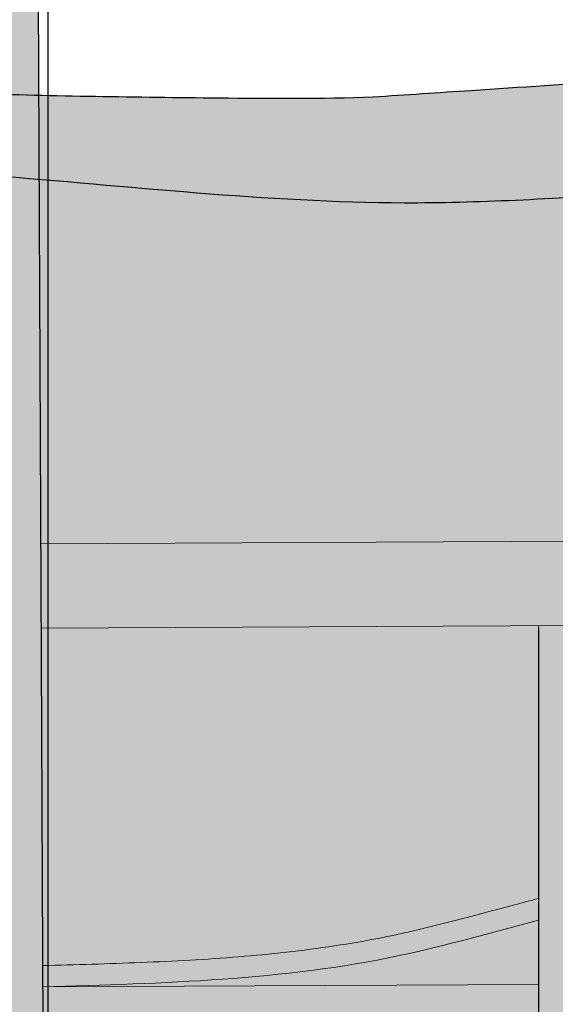
# Model space of a CAD drawing. Units: millimetres. Extents: x 11032 to 26788, y 3406 to 24505.
# Tile 65 of 78: x 18468 to 19737, y 15108 to 17443. Entities that reach past the tile are written whole.
import ezdxf

# ---------------------------------------------------------------- set-up
doc = ezdxf.new("R2010")
doc.units = ezdxf.units.MM
doc.header["$MEASUREMENT"] = 0
for name, color, linetype, lineweight in [('A-ANNO-DIMS', 2, 'Continuous', 18), ('A-ELEV-NECK', 7, 'Continuous', 25), ('A-GLAZ', 250, 'Continuous', 20), ('A-GLAZ-PATT', 9, 'Continuous', 13), ('A-ROOF', 7, 'Continuous', 30), ('E-LITE', 7, 'Continuous', 18), ('E-LITE-PATT', 7, 'Continuous', 13)]:
    doc.layers.add(name, color=color, linetype=linetype, lineweight=lineweight)
for name, color, linetype, lineweight, true_color in [('A-ELEV-NECK-PATT', 159, 'Continuous', 13, 0x22346e), ('A-GLAZ-FRAM-PATT', 250, 'Continuous', 13, 0x262627), ('A-ROOF-PATT', 9, 'Continuous', 13, 0xc7c8ca)]:
    doc.layers.add(name, color=color, linetype=linetype, lineweight=lineweight, true_color=true_color)
doc.styles.get("Standard").update_dxf_attribs({"font": 'arial.ttf'})
doc.dimstyles.get("Standard").update_dxf_attribs({"dimtxt": 150, "dimasz": 100, "dimexe": 10, "dimexo": 5, "dimgap": 5, "dimtad": 0, "dimtih": 1, "dimtoh": 1, "dimdec": 0, "dimzin": 0, "dimdsep": 46, "dimtxsty": 'Standard', "dimcen": 0.09, "dimadec": 0, "dimazin": 0, "dimtfac": 1, "dimtdec": 0, "dimtofl": 0, "dimtmove": 0, "dimatfit": 3, "dimfxl": 1, "dimtolj": 1, "dimtzin": 0, "dimarcsym": 0})

# ---------------------------------------------------------------- blocks, each defined once
blk = doc.blocks.new('*D36')
at = {"layer": 'A-ANNO-DIMS', "color": 0, "lineweight": -2, "transparency": 16777216}
for p, q in [((12301.3, 17115.9), (12301.3, 24416.9)), ((25397.4, 4466.4), (25397.4, 24416.9)), ((12401.3, 24406.9), (18569.2, 24406.9)), ((25297.4, 24406.9), (19129.5, 24406.9))]:
    blk.add_line(p, q, dxfattribs=at)
at = {"layer": 'A-ANNO-DIMS', "color": 0, "transparency": 16777216}
for points in [[(12401.3, 24423.5), (12401.3, 24390.2), (12301.3, 24406.9)], [(25297.4, 24423.5), (25297.4, 24390.2), (25397.4, 24406.9)]]:
    blk.add_solid(points, dxfattribs=at)
at = {"layer": 'Defpoints', "color": 0, "transparency": 16777216}
for p in [(25397.4, 24406.9), (12301.3, 17110.9), (25397.4, 4461.4)]:
    blk.add_point(p, dxfattribs=at)
at = {"layer": 'A-ANNO-DIMS', "color": 0, "transparency": 16777216, "insert": (18849.3, 24406.9), "char_height": 150, "attachment_point": 5}
blk.add_mtext('\\A1;13096', dxfattribs=at)
blk = doc.blocks.new('*D45')
at = {"layer": 'A-ANNO-DIMS', "color": 0, "lineweight": -2, "transparency": 16777216}
for p, q in [((13792.4, 18518.9), (26363.9, 18518.9)), ((26353.9, 18418.9), (26353.9, 17450.3)), ((26353.9, 16318.4), (26353.9, 17287)), ((22902.4, 16218.4), (26363.9, 16218.4))]:
    blk.add_line(p, q, dxfattribs=at)
at = {"layer": 'A-ANNO-DIMS', "color": 0, "transparency": 16777216}
for points in [[(26337.2, 18418.9), (26370.6, 18418.9), (26353.9, 18518.9)], [(26337.2, 16318.4), (26370.6, 16318.4), (26353.9, 16218.4)]]:
    blk.add_solid(points, dxfattribs=at)
at = {"layer": 'Defpoints', "color": 0, "transparency": 16777216}
for p in [(13787.4, 18518.9), (26353.9, 18518.9), (22897.4, 16218.4)]:
    blk.add_point(p, dxfattribs=at)
at = {"layer": 'A-ANNO-DIMS', "color": 0, "transparency": 16777216, "insert": (26353.9, 17368.7), "char_height": 150, "attachment_point": 5}
blk.add_mtext('\\A1;2300.5', dxfattribs=at)
blk = doc.blocks.new('*D50')
at = {"layer": 'A-ANNO-DIMS', "color": 0, "lineweight": -2, "transparency": 16777216}
for p, q in [((19697.4, 16000.7), (19697.4, 3494.9)), ((17953.5, 10206.4), (17953.5, 3494.9)), ((18053.5, 3504.9), (18603.8, 3504.9)), ((19597.4, 3504.9), (19047, 3504.9))]:
    blk.add_line(p, q, dxfattribs=at)
at = {"layer": 'A-ANNO-DIMS', "color": 0, "transparency": 16777216}
for points in [[(18053.5, 3521.6), (18053.5, 3488.2), (17953.5, 3504.9)], [(19597.4, 3521.6), (19597.4, 3488.2), (19697.4, 3504.9)]]:
    blk.add_solid(points, dxfattribs=at)
at = {"layer": 'Defpoints', "color": 0, "transparency": 16777216}
for p in [(19697.4, 16005.7), (17953.5, 10211.4), (19697.4, 3504.9)]:
    blk.add_point(p, dxfattribs=at)
at = {"layer": 'A-ANNO-DIMS', "color": 0, "transparency": 16777216, "insert": (18825.4, 3504.9), "char_height": 150, "attachment_point": 5}
blk.add_mtext('\\A1;1744', dxfattribs=at)
blk = doc.blocks.new('*D51')
at = {"layer": 'A-ANNO-DIMS', "color": 0, "lineweight": -2, "transparency": 16777216}
for p, q in [((19697.4, 16000.7), (19697.4, 3494.9)), ((21997.4, 16011.6), (21997.4, 3494.9)), ((19797.4, 3504.9), (20617.4, 3504.9)), ((21897.4, 3504.9), (21077.4, 3504.9))]:
    blk.add_line(p, q, dxfattribs=at)
at = {"layer": 'A-ANNO-DIMS', "color": 0, "transparency": 16777216}
for points in [[(19797.4, 3521.6), (19797.4, 3488.2), (19697.4, 3504.9)], [(21897.4, 3521.6), (21897.4, 3488.2), (21997.4, 3504.9)]]:
    blk.add_solid(points, dxfattribs=at)
at = {"layer": 'Defpoints', "color": 0, "transparency": 16777216}
for p in [(21997.4, 16016.6), (19697.4, 16005.7), (21997.4, 3504.9)]:
    blk.add_point(p, dxfattribs=at)
at = {"layer": 'A-ANNO-DIMS', "color": 0, "transparency": 16777216, "insert": (20847.4, 3504.9), "char_height": 150, "attachment_point": 5}
blk.add_mtext('\\A1;2300', dxfattribs=at)
blk = doc.blocks.new('*D57')
at = {"layer": 'A-ANNO-DIMS', "color": 0, "lineweight": -2, "transparency": 16777216}
for p, q in [((14994.7, 7266.4), (14994.7, 24416.9)), ((20894.7, 7266.4), (20894.7, 24416.9)), ((15094.7, 24406.9), (17716, 24406.9)), ((20794.7, 24406.9), (18173.4, 24406.9))]:
    blk.add_line(p, q, dxfattribs=at)
at = {"layer": 'A-ANNO-DIMS', "color": 0, "transparency": 16777216}
for points in [[(15094.7, 24423.5), (15094.7, 24390.2), (14994.7, 24406.9)], [(20794.7, 24423.5), (20794.7, 24390.2), (20894.7, 24406.9)]]:
    blk.add_solid(points, dxfattribs=at)
at = {"layer": 'Defpoints', "color": 0, "transparency": 16777216}
for p in [(20894.7, 24406.9), (14994.7, 7261.4), (20894.7, 7261.4)]:
    blk.add_point(p, dxfattribs=at)
at = {"layer": 'A-ANNO-DIMS', "color": 0, "transparency": 16777216, "insert": (17944.7, 24406.9), "char_height": 150, "attachment_point": 5}
blk.add_mtext('\\A1;5900', dxfattribs=at)
blk = doc.blocks.new('*D65')
at = {"layer": 'A-ANNO-DIMS', "color": 0, "lineweight": -2, "transparency": 16777216}
for p, q in [((17362, 12566.3), (17362, 24416.9)), ((18535.4, 12566.5), (18535.4, 24416.9)), ((17462, 24406.9), (17639.4, 24406.9)), ((18435.4, 24406.9), (18258, 24406.9))]:
    blk.add_line(p, q, dxfattribs=at)
at = {"layer": 'A-ANNO-DIMS', "color": 0, "transparency": 16777216}
for points in [[(17462, 24423.5), (17462, 24390.2), (17362, 24406.9)], [(18435.4, 24423.5), (18435.4, 24390.2), (18535.4, 24406.9)]]:
    blk.add_solid(points, dxfattribs=at)
at = {"layer": 'Defpoints', "color": 0, "transparency": 16777216}
for p in [(18535.4, 24406.9), (17362, 12561.3), (18535.4, 12561.5)]:
    blk.add_point(p, dxfattribs=at)
at = {"layer": 'A-ANNO-DIMS', "color": 0, "transparency": 16777216, "insert": (17948.7, 24406.9), "char_height": 150, "attachment_point": 5}
blk.add_mtext('\\A1;1173.3', dxfattribs=at)

msp = doc.modelspace()

# ---------------------------------------------------------------- hatches: boundary and pattern name
at = {"layer": 'A-ELEV-NECK-PATT'}
h = msp.add_hatch(color=256, dxfattribs=at)
h.set_gradient(color1=(82, 15, 16), color2=(153, 76, 0), name='INVHEMISPHERICAL')
edge = h.paths.add_edge_path()
edge.add_line((18055.913, 21712.945), (17991.118, 21712.945))
edge.add_line((17991.118, 21712.945), (17913.235, 17287.655))
edge.add_spline(control_points=[(17913.235, 17287.655), (17923.7, 17287.302), (17934.19, 17286.996), (17944.704, 17286.735)], knot_values=[8963.99017486, 8963.99017486, 8963.99017486, 8963.99017486, 8996.4318779, 8996.4318779, 8996.4318779, 8996.4318779], degree=3, periodic=0)
edge.add_spline(control_points=[(17944.704, 17286.735), (17964.82, 17285.722), (17984.935, 17284.709), (18005.051, 17283.703)], knot_values=[0, 0, 0, 0, 60.41749209, 60.41749209, 60.41749209, 60.41749209], degree=3, periodic=0)
edge.add_line((18005.051, 17283.703), (18055.913, 21712.945))
edge = h.paths.add_edge_path()
edge.add_line((18492.19, 21712.945), (18416.998, 21712.945))
edge.add_line((18416.998, 21712.945), (18420.504, 17266.134))
edge.add_spline(control_points=[(18420.504, 17266.134), (18451.394, 17265.216), (18482.287, 17264.397), (18513.182, 17263.662)], knot_values=[476.26006783, 476.26006783, 476.26006783, 476.26006783, 568.98430855, 568.98430855, 568.98430855, 568.98430855], degree=3, periodic=0)
edge.add_line((18513.182, 17263.662), (18492.19, 21712.945))
edge = h.paths.add_edge_path()
edge.add_spline(control_points=[(18296.914, 17270.367), (18316.656, 17269.603), (18349.518, 17268.396), (18382.383, 17267.313), (18395.503, 17266.9)], knot_values=[352.58081587, 352.58081587, 352.58081587, 352.58081587, 411.85892504, 451.24395945, 451.24395945, 451.24395945, 451.24395945], degree=3, periodic=0)
edge.add_line((18395.503, 17266.9), (18391.999, 21712.945))
edge.add_line((18391.999, 21712.945), (18316.752, 21712.945))
edge.add_line((18316.752, 21712.945), (18296.914, 17270.367))
edge = h.paths.add_edge_path()
edge.add_line((18291.755, 21712.945), (18216.518, 21712.945))
edge.add_line((18216.518, 21712.945), (18173.381, 17275.594))
edge.add_spline(control_points=[(18173.381, 17275.594), (18206.225, 17274.101), (18239.071, 17272.678), (18271.92, 17271.355)], knot_values=[228.93242669, 228.93242669, 228.93242669, 228.93242669, 327.56540209, 327.56540209, 327.56540209, 327.56540209], degree=3, periodic=0)
edge.add_line((18271.92, 17271.355), (18291.755, 21712.945))
h = msp.add_hatch(color=256, dxfattribs=at)
h.set_gradient(color1=(153, 76, 0), color2=(153, 38, 0), name='INVSPHERICAL')
edge = h.paths.add_edge_path()
edge.add_spline(control_points=[(17641.798, 17308.706), (17605.243, 17313.31), (17568.929, 17318.668), (17532.827, 17324.837)], knot_values=[8560.66857913, 8560.66857913, 8560.66857913, 8560.66857913, 8678.18536837, 8678.18536837, 8678.18536837, 8678.18536837], degree=3, periodic=0)
edge.add_line((17532.827, 17324.837), (17525.58, 17122.709))
edge.add_spline(control_points=[(17525.58, 17122.709), (17542.498, 17119.989), (17559.438, 17117.434), (17596.281, 17112.234), (17616.191, 17109.648), (17636.137, 17107.272)], knot_values=[8357.5016646, 8357.5016646, 8357.5016646, 8357.5016646, 8408.27359921, 8408.27359921, 8467.76262378, 8467.76262378, 8467.76262378, 8467.76262378], degree=3, periodic=0)
edge.add_line((17636.137, 17107.272), (17641.798, 17308.706))
edge = h.paths.add_edge_path()
edge.add_spline(control_points=[(17764.917, 17296.043), (17731.975, 17298.702), (17699.249, 17301.903), (17666.718, 17305.687)], knot_values=[8704.84912349, 8704.84912349, 8704.84912349, 8704.84912349, 8809.1081873, 8809.1081873, 8809.1081873, 8809.1081873], degree=3, periodic=0)
edge.add_line((17666.718, 17305.687), (17661.061, 17104.414))
edge.add_spline(control_points=[(17661.061, 17104.414), (17679.29, 17102.404), (17697.549, 17100.566), (17730.647, 17097.538), (17745.476, 17096.292), (17760.326, 17095.15)], knot_values=[8492.52413318, 8492.52413318, 8492.52413318, 8492.52413318, 8546.81227116, 8546.81227116, 8590.76516304, 8590.76516304, 8590.76516304, 8590.76516304], degree=3, periodic=0)
edge.add_line((17760.326, 17095.15), (17764.917, 17296.043))
edge = h.paths.add_edge_path()
edge.add_spline(control_points=[(17785.288, 17093.328), (17818.317, 17091.049), (17851.456, 17089.272), (17884.718, 17087.959)], knot_values=[8615.37173025, 8615.37173025, 8615.37173025, 8615.37173025, 8712.96274361, 8712.96274361, 8712.96274361, 8712.96274361], degree=3, periodic=0)
edge.add_line((17884.718, 17087.959), (17888.249, 17288.59))
edge.add_spline(control_points=[(17888.249, 17288.59), (17855.23, 17289.947), (17822.446, 17291.782), (17789.878, 17294.135)], knot_values=[8835.39626479, 8835.39626479, 8835.39626479, 8835.39626479, 8938.12522047, 8938.12522047, 8938.12522047, 8938.12522047], degree=3, periodic=0)
edge.add_line((17789.878, 17294.135), (17785.288, 17093.328))
edge = h.paths.add_edge_path()
edge.add_spline(control_points=[(17909.705, 17087.059), (17910.273, 17087.04), (17910.841, 17087.022), (17922.493, 17086.648), (17933.591, 17086.342), (17944.704, 17086.084)], knot_values=[8737.37614655, 8737.37614655, 8737.37614655, 8737.37614655, 8739.04043473, 8739.04043473, 8771.49406906, 8771.49406906, 8771.49406906, 8771.49406906], degree=3, periodic=0)
edge.add_spline(control_points=[(17944.704, 17086.084), (17964.06, 17086.958), (17983.426, 17087.583), (18002.804, 17087.985)], knot_values=[1891.03799383, 1891.03799383, 1891.03799383, 1891.03799383, 1949.25960113, 1949.25960113, 1949.25960113, 1949.25960113], degree=3, periodic=0)
edge.add_line((18002.804, 17087.985), (18005.051, 17283.703))
edge.add_spline(control_points=[(18005.051, 17283.703), (17984.935, 17284.709), (17964.82, 17285.722), (17944.704, 17286.735)], knot_values=[0, 0, 0, 0, 60.41749209, 60.41749209, 60.41749209, 60.41749209], degree=3, periodic=0)
edge.add_spline(control_points=[(17944.704, 17286.735), (17934.19, 17286.996), (17923.7, 17287.302), (17913.235, 17287.655)], knot_values=[8963.99017486, 8963.99017486, 8963.99017486, 8963.99017486, 8996.4318779, 8996.4318779, 8996.4318779, 8996.4318779], degree=3, periodic=0)
edge.add_line((17913.235, 17287.655), (17909.705, 17087.059))
edge = h.paths.add_edge_path()
edge.add_spline(control_points=[(18148.395, 17276.742), (18108.941, 17278.575), (18069.489, 17280.497), (18030.038, 17282.457)], knot_values=[85.43243603, 85.43243603, 85.43243603, 85.43243603, 203.92020001, 203.92020001, 203.92020001, 203.92020001], degree=3, periodic=0)
edge.add_line((18030.038, 17282.457), (18027.809, 17088.381))
edge.add_spline(control_points=[(18027.809, 17088.381), (18067.33, 17088.817), (18106.905, 17088.367), (18146.553, 17087.237)], knot_values=[1747.32517671, 1747.32517671, 1747.32517671, 1747.32517671, 1866.00187039, 1866.00187039, 1866.00187039, 1866.00187039], degree=3, periodic=0)
edge.add_line((18146.553, 17087.237), (18148.395, 17276.742))
edge = h.paths.add_edge_path()
edge.add_spline(control_points=[(18271.92, 17271.355), (18239.071, 17272.678), (18206.225, 17274.101), (18173.381, 17275.594)], knot_values=[228.93242669, 228.93242669, 228.93242669, 228.93242669, 327.56540209, 327.56540209, 327.56540209, 327.56540209], degree=3, periodic=0)
edge.add_line((18173.381, 17275.594), (18171.542, 17086.437))
edge.add_spline(control_points=[(18171.542, 17086.437), (18204.662, 17085.263), (18237.835, 17083.647), (18271.073, 17081.706)], knot_values=[1623.3453903, 1623.3453903, 1623.3453903, 1623.3453903, 1722.40133721, 1722.40133721, 1722.40133721, 1722.40133721], degree=3, periodic=0)
edge.add_line((18271.073, 17081.706), (18271.92, 17271.355))
edge = h.paths.add_edge_path()
edge.add_spline(control_points=[(18296.064, 17080.189), (18329.191, 17078.104), (18362.384, 17075.728), (18395.656, 17073.18)], knot_values=[1499.9078295, 1499.9078295, 1499.9078295, 1499.9078295, 1598.53123513, 1598.53123513, 1598.53123513, 1598.53123513], degree=3, periodic=0)
edge.add_line((18395.656, 17073.18), (18395.503, 17266.9))
edge.add_spline(control_points=[(18395.503, 17266.9), (18382.383, 17267.313), (18349.518, 17268.396), (18316.656, 17269.603), (18296.914, 17270.367)], knot_values=[352.58081587, 352.58081587, 352.58081587, 352.58081587, 391.96585028, 451.24395945, 451.24395945, 451.24395945, 451.24395945], degree=3, periodic=0)
edge.add_line((18296.914, 17270.367), (18296.064, 17080.189))
edge = h.paths.add_edge_path()
edge.add_spline(control_points=[(18420.658, 17071.235), (18423.571, 17071.005), (18454.665, 17068.542), (18485.83, 17065.963), (18514.126, 17063.566)], knot_values=[1383.18424693, 1383.18424693, 1383.18424693, 1383.18424693, 1391.81011968, 1475.21962479, 1475.21962479, 1475.21962479, 1475.21962479], degree=3, periodic=0)
edge.add_line((18514.126, 17063.566), (18513.182, 17263.662))
edge.add_spline(control_points=[(18513.182, 17263.662), (18482.287, 17264.397), (18451.394, 17265.216), (18420.504, 17266.134)], knot_values=[476.26006783, 476.26006783, 476.26006783, 476.26006783, 568.98430855, 568.98430855, 568.98430855, 568.98430855], degree=3, periodic=0)
edge.add_line((18420.504, 17266.134), (18420.658, 17071.235))
h = msp.add_hatch(color=256, dxfattribs=at)
h.set_gradient(color1=(82, 15, 16), color2=(153, 76, 0), name='INVHEMISPHERICAL')
edge = h.paths.add_edge_path()
edge.add_line((17829.868, 12550.781), (17950.703, 12550.781))
edge.add_line((17950.703, 12550.781), (18002.804, 17087.985))
edge.add_spline(control_points=[(18002.804, 17087.985), (17983.426, 17087.583), (17964.06, 17086.958), (17944.704, 17086.084)], knot_values=[1891.03799383, 1891.03799383, 1891.03799383, 1891.03799383, 1949.25960113, 1949.25960113, 1949.25960113, 1949.25960113], degree=3, periodic=0)
edge.add_spline(control_points=[(17944.704, 17086.084), (17933.591, 17086.342), (17922.493, 17086.648), (17910.841, 17087.022), (17910.273, 17087.04), (17909.705, 17087.059)], knot_values=[8737.37614655, 8737.37614655, 8737.37614655, 8737.37614655, 8769.82978089, 8769.82978089, 8771.49406906, 8771.49406906, 8771.49406906, 8771.49406906], degree=3, periodic=0)
edge.add_line((17909.705, 17087.059), (17829.868, 12550.781))
edge = h.paths.add_edge_path()
edge.add_spline(control_points=[(18146.553, 17087.237), (18106.905, 17088.367), (18067.33, 17088.817), (18027.809, 17088.381)], knot_values=[1747.32517671, 1747.32517671, 1747.32517671, 1747.32517671, 1866.00187039, 1866.00187039, 1866.00187039, 1866.00187039], degree=3, periodic=0)
edge.add_line((18027.809, 17088.381), (17975.703, 12550.781))
edge.add_line((17975.703, 12550.781), (18102.451, 12550.781))
edge.add_line((18102.451, 12550.781), (18146.553, 17087.237))
edge = h.paths.add_edge_path()
edge.add_line((18127.45, 12550.781), (18250.839, 12550.781))
edge.add_line((18250.839, 12550.781), (18271.073, 17081.706))
edge.add_spline(control_points=[(18271.073, 17081.706), (18237.835, 17083.647), (18204.662, 17085.263), (18171.542, 17086.437)], knot_values=[1623.3453903, 1623.3453903, 1623.3453903, 1623.3453903, 1722.40133721, 1722.40133721, 1722.40133721, 1722.40133721], degree=3, periodic=0)
edge.add_line((18171.542, 17086.437), (18127.45, 12550.781))
edge = h.paths.add_edge_path()
edge.add_spline(control_points=[(18395.656, 17073.18), (18362.384, 17075.728), (18329.191, 17078.104), (18296.064, 17080.189)], knot_values=[1499.9078295, 1499.9078295, 1499.9078295, 1499.9078295, 1598.53123513, 1598.53123513, 1598.53123513, 1598.53123513], degree=3, periodic=0)
edge.add_line((18296.064, 17080.189), (18275.839, 12550.781))
edge.add_line((18275.839, 12550.781), (18399.221, 12550.781))
edge.add_line((18399.221, 12550.781), (18395.656, 17073.18))
edge = h.paths.add_edge_path()
edge.add_spline(control_points=[(18514.126, 17063.566), (18485.83, 17065.963), (18454.665, 17068.542), (18423.571, 17071.005), (18420.658, 17071.235)], knot_values=[1383.18424693, 1383.18424693, 1383.18424693, 1383.18424693, 1466.59375204, 1475.21962479, 1475.21962479, 1475.21962479, 1475.21962479], degree=3, periodic=0)
edge.add_line((18420.658, 17071.235), (18424.221, 12551.892))
edge.add_line((18424.221, 12551.892), (18535.368, 12561.343))
edge.add_line((18535.368, 12561.343), (18514.126, 17063.566))
edge = h.paths.add_edge_path()
edge.add_spline(control_points=[(17636.137, 17107.272), (17616.191, 17109.648), (17596.281, 17112.234), (17559.438, 17117.434), (17542.498, 17119.989), (17525.58, 17122.709)], knot_values=[8357.5016646, 8357.5016646, 8357.5016646, 8357.5016646, 8416.99068917, 8416.99068917, 8467.76262378, 8467.76262378, 8467.76262378, 8467.76262378], degree=3, periodic=0)
edge.add_line((17525.58, 17122.709), (17362.033, 12561.3))
edge.add_line((17362.033, 12561.3), (17485.63, 12550.781))
edge.add_line((17485.63, 12550.781), (17508.079, 12550.781))
edge.add_line((17508.079, 12550.781), (17636.137, 17107.272))
edge = h.paths.add_edge_path()
edge.add_spline(control_points=[(17760.326, 17095.15), (17745.476, 17096.292), (17730.647, 17097.538), (17697.549, 17100.566), (17679.29, 17102.404), (17661.061, 17104.414)], knot_values=[8492.52413318, 8492.52413318, 8492.52413318, 8492.52413318, 8536.47702506, 8536.47702506, 8590.76516304, 8590.76516304, 8590.76516304, 8590.76516304], degree=3, periodic=0)
edge.add_line((17661.061, 17104.414), (17533.08, 12550.781))
edge.add_line((17533.08, 12550.781), (17656.474, 12550.781))
edge.add_line((17656.474, 12550.781), (17760.326, 17095.15))
edge = h.paths.add_edge_path()
edge.add_spline(control_points=[(17884.718, 17087.959), (17851.456, 17089.272), (17818.317, 17091.049), (17785.288, 17093.328)], knot_values=[8615.37173025, 8615.37173025, 8615.37173025, 8615.37173025, 8712.96274361, 8712.96274361, 8712.96274361, 8712.96274361], degree=3, periodic=0)
edge.add_line((17785.288, 17093.328), (17681.475, 12550.781))
edge.add_line((17681.475, 12550.781), (17804.868, 12550.781))
edge.add_line((17804.868, 12550.781), (17884.718, 17087.959))
at = {"layer": 'A-GLAZ-FRAM-PATT'}
h = msp.add_hatch(color=256, dxfattribs=at)
h.paths.add_polyline_path([(22747.404, 16218.44), (22395.025, 16218.44), (18518.2, 16200.148), (18519.143, 16000.151), (22747.404, 16020.1)])
edge = h.paths.add_edge_path()
edge.add_line((22897.404, 16218.44), (22747.404, 16218.44))
edge.add_line((22747.404, 16218.44), (22747.404, 16020.1))
edge.add_line((22747.404, 16020.1), (22747.404, 9631.346))
edge.add_spline(control_points=[(22747.404, 9631.346), (22803.273, 9520.228), (22853.467, 9405.87), (22897.404, 9289.211)], knot_values=[2645.78092422, 2645.78092422, 2645.78092422, 2645.78092422, 3013.05623672, 3013.05623672, 3013.05623672, 3013.05623672], degree=3, periodic=0)
edge.add_line((22897.404, 9289.211), (22897.404, 16218.44))
h.paths.add_polyline_path([(22097.404, 16017.033), (21997.404, 16016.562), (21997.404, 13316.532), (22097.404, 13317.003)])
edge = h.paths.add_edge_path()
edge.add_line((19797.404, 16006.182), (19697.404, 16005.71))
edge.add_line((19697.404, 16005.71), (19697.404, 15155.703))
edge.add_line((19697.404, 15155.703), (19697.404, 12747.012))
edge.add_spline(control_points=[(19697.404, 12747.012), (19708.389, 12750.081), (19719.253, 12753.406), (19732.457, 12757.789), (19734.918, 12758.62), (19737.372, 12759.464)], knot_values=[1372.60477099, 1372.60477099, 1372.60477099, 1372.60477099, 1399.44343377, 1399.44343377, 1405.61279972, 1405.61279972, 1405.61279972, 1405.61279972], degree=3, periodic=0)
edge.add_spline(control_points=[(19737.372, 12759.464), (19750.245, 12763.891), (19762.932, 12768.657), (19778.9, 12775.14), (19782.354, 12776.572), (19785.794, 12778.028)], knot_values=[1405.61279972, 1405.61279972, 1405.61279972, 1405.61279972, 1437.96891336, 1437.96891336, 1446.94640473, 1446.94640473, 1446.94640473, 1446.94640473], degree=3, periodic=0)
edge.add_spline(control_points=[(19785.794, 12778.028), (19789.682, 12779.673), (19793.552, 12781.348), (19797.404, 12783.051)], knot_values=[1446.94640473, 1446.94640473, 1446.94640473, 1446.94640473, 1457.09545574, 1457.09545574, 1457.09545574, 1457.09545574], degree=3, periodic=0)
edge.add_line((19797.404, 12783.051), (19797.404, 15306.174))
edge.add_line((19797.404, 15306.174), (19797.404, 16006.182))
h = msp.add_hatch(color=256, dxfattribs=at)
h.paths.add_polyline_path([(19697.404, 15155.703), (18523.154, 15150.163), (18523.626, 15050.164), (19697.404, 15055.702)])
h.paths.add_polyline_path([(21997.404, 15166.555), (19797.404, 15156.175), (19797.404, 15056.174), (20912.335, 15061.434, -0.11801722), (20947.253, 15061.599), (21997.404, 15066.554)])
h.paths.add_polyline_path([(22747.404, 15170.094), (22097.404, 15167.027), (22097.404, 15067.026), (22747.404, 15070.092)])
edge = h.paths.add_edge_path()
edge.add_line((21997.404, 13241.531), (21332.397, 13238.393))
edge.add_spline(control_points=[(21332.397, 13238.393), (21338.038, 13214.902), (21343.139, 13191.382), (21354.5, 13132.481), (21360.029, 13097.149), (21368.306, 13027.119), (21371.052, 12992.421), (21373.63, 12924.101), (21373.462, 12890.481), (21370.61, 12834.187), (21368.665, 12811.15), (21365.955, 12788.546)], knot_values=[4470.65028407, 4470.65028407, 4470.65028407, 4470.65028407, 4531.4505555, 4531.4505555, 4623.16319106, 4623.16319106, 4714.87582662, 4714.87582662, 4806.58846218, 4806.58846218, 4871.89074498, 4871.89074498, 4871.89074498, 4871.89074498], degree=3, periodic=0)
edge.add_line((21365.955, 12788.546), (21997.404, 12791.526))
edge.add_line((21997.404, 12791.526), (21997.404, 13241.531))
h.paths.add_polyline_path([(22097.404, 13242.003), (21997.404, 13241.531), (21997.404, 12791.526), (22097.404, 12791.998)])
h.paths.add_polyline_path([(22697.404, 13244.833), (22097.404, 13242.003), (22097.404, 12791.998), (22697.404, 12794.828)])
at = {"layer": 'A-GLAZ-PATT'}
h = msp.add_hatch(color=256, dxfattribs=at)
h.set_gradient(color1=(254, 221, 154), color2=(248, 246, 176), name='CURVED')
edge = h.paths.add_edge_path()
edge.add_spline(control_points=[(18522.918, 15200.175), (18561.599, 15201.209), (18600.224, 15202.243), (18716.594, 15205.749), (18794.099, 15208.613), (18948.086, 15217.451), (19024.568, 15223.425), (19176.135, 15240.511), (19251.219, 15251.623), (19333.848, 15267.966), (19342.25, 15269.676), (19356.967, 15272.758), (19363.289, 15274.111), (19375.94, 15276.871), (19382.267, 15278.279), (19401.252, 15282.576), (19413.915, 15285.541), (19451.935, 15294.685), (19477.322, 15301.111), (19548.254, 15319.552), (19593.948, 15331.984), (19659.079, 15349.253), (19678.203, 15354.269), (19697.404, 15359.188)], knot_values=[1.09285599, 1.09285599, 1.09285599, 1.09285599, 116.34451384, 116.34451384, 349.03354152, 349.03354152, 581.72256921, 581.72256921, 814.41159689, 814.41159689, 840.78637359, 840.78637359, 860.67891922, 860.67891922, 880.57146485, 880.57146485, 920.35655611, 920.35655611, 999.92673863, 999.92673863, 1142.09604805, 1142.09604805, 1200.90860694, 1200.90860694, 1200.90860694, 1200.90860694], degree=3, periodic=0)
edge.add_line((19697.404, 15359.188), (19697.404, 16005.71))
edge.add_line((19697.404, 16005.71), (18519.143, 16000.151))
edge.add_line((18519.143, 16000.151), (18522.918, 15200.175))
edge = h.paths.add_edge_path()
edge.add_line((19697.404, 15055.702), (18523.626, 15050.164))
edge.add_line((18523.626, 15050.164), (18531.851, 13306.733))
edge.add_spline(control_points=[(18531.851, 13306.733), (18553.325, 13284.933), (18574.901, 13263.301), (18632.771, 13206.214), (18669.261, 13171.188), (18735.852, 13109.762), (18765.813, 13083.011), (18826.398, 13031.156), (18857.021, 13006.052), (18919.15, 12957.862), (18950.655, 12934.774), (19007.615, 12895.967), (19032.834, 12879.759), (19084.165, 12849.05), (19110.278, 12834.547), (19163.6, 12807.555), (19190.811, 12795.065), (19240.068, 12775.123), (19261.85, 12767.175), (19306.233, 12752.949), (19328.834, 12746.672), (19374.859, 12736.071), (19398.283, 12731.748), (19445.866, 12725.365), (19470.026, 12723.306), (19514.597, 12721.889), (19534.921, 12722.121), (19575.756, 12724.466), (19596.267, 12726.579), (19622.683, 12730.57), (19628.6, 12731.546), (19638.601, 12733.337), (19642.688, 12734.108), (19650.826, 12735.723), (19654.881, 12736.567), (19667.001, 12739.207), (19675.023, 12741.111), (19687.813, 12744.388), (19692.62, 12745.676), (19697.404, 12747.012)], knot_values=[259.28299856, 259.28299856, 259.28299856, 259.28299856, 332.45020059, 332.45020059, 454.53383699, 454.53383699, 552.84889009, 552.84889009, 651.16394319, 651.16394319, 749.47899629, 749.47899629, 825.6298474, 825.6298474, 901.7806985, 901.7806985, 977.9315496, 977.9315496, 1036.43952646, 1036.43952646, 1094.94750331, 1094.94750331, 1153.45548017, 1153.45548017, 1211.96345702, 1211.96345702, 1260.21270617, 1260.21270617, 1308.46195531, 1308.46195531, 1322.39247458, 1322.39247458, 1332.02384448, 1332.02384448, 1341.65521438, 1341.65521438, 1360.91795418, 1360.91795418, 1372.60477099, 1372.60477099, 1372.60477099, 1372.60477099], degree=3, periodic=0)
edge.add_line((19697.404, 12747.012), (19697.404, 15055.702))
h.paths.add_polyline_path([(18790.086, 14298.34, -1), (18890.086, 14298.34, -1)], flags=16)
h.paths.add_polyline_path([(19437.524, 14550.125, -1), (19537.524, 14550.125, -1)], flags=16)
h.paths.add_polyline_path([(22697.404, 16019.864), (22097.404, 16017.033), (22097.404, 15167.027), (22697.404, 15169.858)])
h.paths.add_polyline_path([(22697.404, 15069.857), (22097.404, 15067.026), (22097.404, 13317.003), (22697.404, 13319.834)])
h.paths.add_polyline_path([(20866.429, 15795.606, -1), (21016.429, 15795.606, -1)], flags=16)
h.paths.add_polyline_path([(19822.441, 15337.78), (19797.404, 15332.147), (19797.404, 15156.175), (20721.869, 15160.537), (20700.803, 15175.665), (20679.512, 15190.548), (20657.993, 15205.143), (20636.247, 15219.41), (20614.273, 15233.307), (20592.07, 15246.794), (20569.639, 15259.829), (20546.978, 15272.372), (20524.088, 15284.38), (20500.968, 15295.814), (20477.616, 15306.631), (20454.034, 15316.792), (20430.219, 15326.254), (20406.173, 15334.976), (20381.894, 15342.919), (20357.382, 15350.039), (20332.636, 15356.297), (20307.662, 15361.667), (20282.483, 15366.173), (20257.125, 15369.849), (20231.617, 15372.729), (20205.984, 15374.847), (20180.253, 15376.236), (20154.451, 15376.931), (20128.605, 15376.964), (20102.742, 15376.37), (20076.889, 15375.183), (20051.072, 15373.436), (20025.318, 15371.163), (19999.653, 15368.398), (19974.087, 15365.173), (19948.614, 15361.516), (19923.228, 15357.456), (19897.924, 15353.024), (19872.695, 15348.248), (19847.536, 15343.157)])
h.paths.add_polyline_path([(19797.404, 15383.428), (19822.666, 15388.998), (19848.044, 15394.311), (19873.542, 15399.338), (19899.168, 15404.048), (19924.927, 15408.41), (19950.824, 15412.396), (19976.865, 15415.972), (20003.054, 15419.109), (20029.394, 15421.774), (20055.871, 15423.934), (20082.461, 15425.553), (20109.142, 15426.594), (20135.888, 15427.02), (20162.676, 15426.794), (20189.481, 15425.88), (20216.28, 15424.237), (20243.046, 15421.828), (20269.754, 15418.614), (20296.377, 15414.554), (20322.887, 15409.61), (20349.254, 15403.74), (20375.368, 15396.947), (20401.163, 15389.283), (20426.64, 15380.795), (20451.799, 15371.531), (20476.643, 15361.538), (20501.172, 15350.863), (20525.391, 15339.55), (20549.302, 15327.645), (20572.91, 15315.192), (20596.218, 15302.234), (20619.229, 15288.816), (20641.948, 15274.978), (20664.378, 15260.764), (20686.523, 15246.215), (20708.386, 15231.373), (20729.97, 15216.279), (20751.277, 15200.974), (20806.33, 15160.935), (21997.404, 15166.555), (21997.404, 16016.562), (19797.404, 16006.182)])
at = {"layer": 'A-ROOF-PATT'}
h = msp.add_hatch(color=256, dxfattribs=at)
edge = h.paths.add_edge_path()
edge.add_spline(control_points=[(18514.126, 17063.566), (18809.773, 17038.521), (19288.07, 16988.339), (19761.843, 17020.464), (19965.955, 17031.58)], knot_values=[0, 0, 0, 0, 871.48115533, 1383.18424693, 1383.18424693, 1383.18424693, 1383.18424693], degree=3, periodic=0)
edge.add_spline(control_points=[(19965.955, 17031.58), (20122.484, 17046.068), (20408.011, 17091.181), (20910.567, 17150.246), (21440.234, 17310.172), (21915.866, 17351.508), (22364.272, 17406.622), (22705.353, 17409.356), (22912.577, 17410.967), (22981.194, 17409.426)], knot_values=[0, 0, 0, 0, 414.81784697, 1085.22788952, 1556.54039253, 2003.31216232, 2520.51919616, 2899.47011217, 3092.27759325, 3092.27759325, 3092.27759325, 3092.27759325], degree=3, periodic=0)
edge.add_spline(control_points=[(22981.194, 17409.426), (23026.355, 17412.719), (23070.675, 17406.134), (23179.968, 17412.17), (23244.326, 17403.734), (23304.873, 17403.391)], knot_values=[11756.28081343, 11756.28081343, 11756.28081343, 11756.28081343, 11879.15309498, 11879.15309498, 12065.87545546, 12065.87545546, 12065.87545546, 12065.87545546], degree=3, periodic=0)
edge.add_spline(control_points=[(23304.873, 17403.391), (23443.416, 17391.278), (23687.5, 17400.339), (23988.629, 17323.661), (24193.084, 17226.949), (24257.37, 17136.735), (24279.347, 17098.191)], knot_values=[0, 0, 0, 0, 412.75172359, 727.19040018, 931.86025321, 1064.01641738, 1064.01641738, 1064.01641738, 1064.01641738], degree=3, periodic=0)
edge.add_spline(control_points=[(24279.347, 17098.191), (24276.632, 17112.026), (24103.56, 17784.539), (21679.83, 17482.933), (20092.886, 17311.864), (19886.51, 17298.161)], knot_values=[9435.32329041, 9435.32329041, 9435.32329041, 9435.32329041, 9511.54858978, 13244.41643911, 13837.11981978, 13837.11981978, 13837.11981978, 13837.11981978], degree=3, periodic=0)
edge.add_spline(control_points=[(19886.51, 17298.161), (19770.33, 17290.447), (19654.15, 17282.732), (19537.97, 17275.018), (19460.41, 17269.868), (19382.851, 17264.718), (19305.291, 17259.568)], knot_values=[8878.9087223, 8878.9087223, 8878.9087223, 8878.9087223, 9212.57342317, 9212.57342317, 9212.57342317, 9435.32303857, 9435.32303857, 9435.32303857, 9435.32303857], degree=3, periodic=0)
edge.add_spline(control_points=[(19305.291, 17259.568), (19183.371, 17255.041), (18919.19, 17257.277), (18655.158, 17260.282), (18513.182, 17263.662)], knot_values=[568.98430855, 568.98430855, 568.98430855, 568.98430855, 934.97323186, 1361.07600794, 1361.07600794, 1361.07600794, 1361.07600794], degree=3, periodic=0)
edge.add_line((18513.182, 17263.662), (18514.126, 17063.566))
h = msp.add_hatch(color=256, dxfattribs=at)
h.set_gradient(color1=(254, 234, 185), color2=(254, 204, 102), name='HEMISPHERICAL')
edge = h.paths.add_edge_path()
edge.add_line((22395.025, 16218.44), (22897.404, 16218.44))
edge.add_line((22897.404, 16218.44), (22897.404, 14361.22))
edge.add_spline(control_points=[(22897.404, 14361.22), (23633.498, 15762.375), (24369.592, 16638.387), (24279.347, 17098.191)], knot_values=[13837.11981978, 13837.11981978, 13837.11981978, 13837.11981978, 16370.50452639, 16370.50452639, 16370.50452639, 16370.50452639], degree=3, periodic=0)
edge.add_spline(control_points=[(24279.347, 17098.191), (24257.37, 17136.735), (24193.084, 17226.949), (23988.629, 17323.661), (23687.5, 17400.339), (23443.416, 17391.278), (23304.873, 17403.391)], knot_values=[0, 0, 0, 0, 132.15616417, 336.8260172, 651.2646938, 1064.01641738, 1064.01641738, 1064.01641738, 1064.01641738], degree=3, periodic=0)
edge.add_spline(control_points=[(23304.873, 17403.391), (23244.326, 17403.734), (23179.968, 17412.17), (23070.675, 17406.134), (23026.355, 17412.719), (22981.194, 17409.426)], knot_values=[11756.28081343, 11756.28081343, 11756.28081343, 11756.28081343, 11943.0031739, 11943.0031739, 12065.87545546, 12065.87545546, 12065.87545546, 12065.87545546], degree=3, periodic=0)
edge.add_spline(control_points=[(22981.194, 17409.426), (22912.577, 17410.967), (22705.353, 17409.356), (22364.272, 17406.622), (21915.866, 17351.508), (21440.234, 17310.172), (20910.567, 17150.246), (20408.011, 17091.181), (20122.484, 17046.068), (19965.955, 17031.58)], knot_values=[0, 0, 0, 0, 192.80748108, 571.75839709, 1088.96543094, 1535.73720072, 2007.04970373, 2677.45974628, 3092.27759325, 3092.27759325, 3092.27759325, 3092.27759325], degree=3, periodic=0)
edge.add_spline(control_points=[(19965.955, 17031.58), (19761.843, 17020.464), (19288.07, 16988.339), (18809.773, 17038.521), (18514.126, 17063.566)], knot_values=[0, 0, 0, 0, 511.7030916, 1383.18424693, 1383.18424693, 1383.18424693, 1383.18424693], degree=3, periodic=0)
edge.add_line((18514.126, 17063.566), (18518.2, 16200.148))
edge.add_line((18518.2, 16200.148), (22395.025, 16218.44))
h.paths.add_polyline_path([(20159.481, 16629.671, -1), (20359.481, 16629.671, -1)], flags=16)
h.paths.add_polyline_path([(22641.869, 16640.848, -1), (22441.869, 16640.848, -1)], flags=16)
h.paths.add_polyline_path([(23436.23, 16026.079, -1), (23236.23, 16026.079, -1)], flags=16)
at = {"layer": 'E-LITE-PATT'}
h = msp.add_hatch(color=256, dxfattribs=at)
edge = h.paths.add_edge_path()
edge.add_spline(control_points=[(18523.154, 15150.163), (18807.347, 15157.761), (19206.112, 15168.423), (19587.098, 15279.026), (19697.404, 15307.557)], knot_values=[0, 0, 0, 0, 846.75149574, 1188.1141131, 1188.1141131, 1188.1141131, 1188.1141131], degree=3, periodic=0)
edge.add_line((19697.404, 15307.557), (19697.404, 15359.188))
edge.add_spline(control_points=[(19697.404, 15359.188), (19678.203, 15354.269), (19659.079, 15349.253), (19593.948, 15331.984), (19548.254, 15319.552), (19477.322, 15301.111), (19451.935, 15294.685), (19413.915, 15285.541), (19401.252, 15282.576), (19382.267, 15278.279), (19375.94, 15276.871), (19363.289, 15274.111), (19356.967, 15272.758), (19342.25, 15269.676), (19333.848, 15267.966), (19251.219, 15251.623), (19176.135, 15240.511), (19024.568, 15223.425), (18948.086, 15217.451), (18794.099, 15208.613), (18716.594, 15205.749), (18600.224, 15202.243), (18561.599, 15201.209), (18522.918, 15200.175)], knot_values=[1.09285599, 1.09285599, 1.09285599, 1.09285599, 59.90541488, 59.90541488, 202.0747243, 202.0747243, 281.64490682, 281.64490682, 321.42999808, 321.42999808, 341.32254371, 341.32254371, 361.21508934, 361.21508934, 387.58986604, 387.58986604, 620.27889372, 620.27889372, 852.96792141, 852.96792141, 1085.65694909, 1085.65694909, 1200.90860694, 1200.90860694, 1200.90860694, 1200.90860694], degree=3, periodic=0)
edge.add_line((18522.918, 15200.175), (18523.154, 15150.163))
edge = h.paths.add_edge_path()
edge.add_spline(control_points=[(19797.404, 15332.147), (19868.636, 15348.527), (20045.965, 15382.128), (20379.232, 15379.049), (20603.72, 15246.463), (20721.869, 15160.537)], knot_values=[1290.96802179, 1290.96802179, 1290.96802179, 1290.96802179, 1509.98304384, 1831.38750258, 2265.00925431, 2265.00925431, 2265.00925431, 2265.00925431], degree=3, periodic=0)
edge.add_line((20721.869, 15160.537), (20806.33, 15160.935))
edge.add_spline(control_points=[(20806.33, 15160.935), (20787.979, 15174.281), (20769.629, 15187.627), (20751.278, 15200.973), (20751.278, 15200.973), (20751.277, 15200.974), (20751.277, 15200.974)], knot_values=[2265.00925431, 2265.00925431, 2265.00925431, 2265.00925431, 2330.89307837, 2330.89307837, 2330.89307837, 2330.89358007, 2330.89358007, 2330.89358007, 2330.89358007], degree=3, periodic=0)
edge.add_spline(control_points=[(20751.277, 15200.974), (20751.247, 15200.996), (20751.217, 15201.018), (20722.252, 15222.081), (20692.553, 15242.645), (20631.556, 15281.877), (20600.258, 15300.544), (20535.977, 15335.007), (20502.992, 15350.803), (20448.844, 15372.942), (20428.246, 15380.535), (20396.869, 15390.701), (20386.329, 15393.886), (20370.401, 15398.335), (20365.072, 15399.763), (20354.373, 15402.506), (20349.001, 15403.822), (20337.544, 15406.494), (20331.459, 15407.834), (20315.169, 15411.216), (20304.944, 15413.125), (20281.909, 15416.972), (20269.086, 15418.802), (20222.263, 15424.425), (20188.116, 15426.504), (20124.362, 15427.321), (20094.738, 15426.456), (20050.592, 15423.632), (20035.925, 15422.435), (20006.724, 15419.587), (19992.193, 15417.937), (19959.175, 15413.705), (19940.732, 15410.994), (19880.215, 15401.109), (19838.589, 15392.722), (19797.404, 15383.428)], knot_values=[1302.24166378, 1302.24166378, 1302.24166378, 1302.24166378, 1302.35087893, 1302.35087893, 1406.225269, 1406.225269, 1510.09965908, 1510.09965908, 1613.97404916, 1613.97404916, 1676.17986117, 1676.17986117, 1707.28276717, 1707.28276717, 1722.83422018, 1722.83422018, 1738.38567318, 1738.38567318, 1755.91676333, 1755.91676333, 1785.22951081, 1785.22951081, 1821.79065604, 1821.79065604, 1918.47644845, 1918.47644845, 2002.64679624, 2002.64679624, 2044.73197014, 2044.73197014, 2086.81714404, 2086.81714404, 2140.81625119, 2140.81625119, 2265.00925431, 2265.00925431, 2265.00925431, 2265.00925431], degree=3, periodic=0)
edge.add_line((19797.404, 15383.428), (19797.404, 15332.147))
h.paths.add_polyline_path([(21016.429, 15795.606, 1), (20866.429, 15795.606, 1)])
h.paths.add_polyline_path([(23236.23, 16026.079, 1), (23436.23, 16026.079, 1)])
h.paths.add_polyline_path([(22441.869, 16640.848, 1), (22641.869, 16640.848, 1)])
h.paths.add_polyline_path([(20159.481, 16629.671, 1), (20359.481, 16629.671, 1)])
h = msp.add_hatch(color=256, dxfattribs=at)
edge = h.paths.add_edge_path()
edge.add_line((19697.404, 15305.702), (19697.404, 15307.557))
edge.add_spline(control_points=[(19697.404, 15307.557), (19587.098, 15279.026), (19206.112, 15168.423), (18807.347, 15157.761), (18523.154, 15150.163)], knot_values=[0, 0, 0, 0, 341.36261736, 1188.1141131, 1188.1141131, 1188.1141131, 1188.1141131], degree=3, periodic=0)
edge.add_line((18523.154, 15150.163), (19697.404, 15155.703))
edge.add_line((19697.404, 15155.703), (19697.404, 15305.702))

# ---------------------------------------------------------------- linework, layer by layer
at = {"layer": 'A-ELEV-NECK'}
msp.add_line((18535.612, 12509.736), (18492.19, 21712.945), dxfattribs=at)
at = {"layer": 'A-GLAZ'}
for p, q in [((22395.025, 16218.44), (18518.2, 16200.148)), ((22747.404, 16020.1), (18519.143, 16000.151)), ((19697.404, 16005.71), (19697.404, 15155.703)), ((19697.404, 15305.702), (19697.404, 12747.012)), ((19697.404, 15155.703), (18521.974, 15150.157))]:
    msp.add_line(p, q, dxfattribs=at)
at = {"layer": 'A-ROOF'}
for points, knots in [([(19305.291, 17259.568), (19382.851, 17264.718), (19460.41, 17269.868), (19537.97, 17275.018), (19654.15, 17282.732), (19770.33, 17290.447), (19886.51, 17298.161), (19886.51, 17298.161), (19886.51, 17298.161), (19886.51, 17298.161), (20092.886, 17311.864), (21679.83, 17482.933), (25498.5, 17958.124), (23655.645, 15804.534), (22897.404, 14361.22)], [8878.9087223, 8878.9087223, 8878.9087223, 8878.9087223, 9101.65833771, 9101.65833771, 9101.65833771, 9435.32303857, 9435.32303857, 9435.32303857, 9435.32329041, 9435.32329041, 9435.32329041, 10028.02667108, 13760.8945204, 16370.50452639, 16370.50452639, 16370.50452639, 16370.50452639]), ([(17773.744, 17295.344), (17779.125, 17295.073), (17784.506, 17294.802), (17789.887, 17294.531), (17822.68, 17292.88), (17855.473, 17291.228), (17888.266, 17289.577), (17896.593, 17289.157), (17904.92, 17288.738), (17913.247, 17288.319), (17923.732, 17287.791), (17934.218, 17287.263), (17944.704, 17286.735), (18081.831, 17279.829), (18413.143, 17263.145), (18866.785, 17257.721), (19183.371, 17255.041), (19305.291, 17259.568)], [-171.15751174, -171.15751174, -171.15751174, -171.15751174, -154.99648673, -154.99648673, -154.99648673, -56.50264353, -56.50264353, -56.50264353, -31.49350773, -31.49350773, -31.49350773, 0, 0, 0, 411.85892504, 995.08708463, 1361.07600794, 1361.07600794, 1361.07600794, 1361.07600794]), ([(19965.955, 17031.58), (19761.843, 17020.464), (19259.5, 16986.401), (18585.074, 17064.116), (18105.171, 17093.325), (17944.704, 17086.084)], [0, 0, 0, 0, 511.7030916, 1466.59375204, 1949.25960113, 1949.25960113, 1949.25960113, 1949.25960113])]:
    msp.add_open_spline(points, degree=3, knots=knots, dxfattribs=at)
at = {"layer": 'E-LITE'}
for points, knots in [([(18521.818, 15200.145), (18560.866, 15201.189), (18599.858, 15202.232), (18716.594, 15205.749), (18794.099, 15208.613), (18948.086, 15217.451), (19024.568, 15223.425), (19176.135, 15240.511), (19251.219, 15251.623), (19333.848, 15267.966), (19342.25, 15269.676), (19356.967, 15272.758), (19363.289, 15274.111), (19375.94, 15276.871), (19382.267, 15278.279), (19401.252, 15282.576), (19413.915, 15285.541), (19451.935, 15294.685), (19477.322, 15301.111), (19548.254, 15319.552), (19593.948, 15331.984), (19659.079, 15349.253), (19678.203, 15354.269), (19697.404, 15359.188)], [0, 0, 0, 0, 116.34451384, 116.34451384, 349.03354152, 349.03354152, 581.72256921, 581.72256921, 814.41159689, 814.41159689, 840.78637359, 840.78637359, 860.67891922, 860.67891922, 880.57146485, 880.57146485, 920.35655611, 920.35655611, 999.92673863, 999.92673863, 1142.09604805, 1142.09604805, 1200.90860694, 1200.90860694, 1200.90860694, 1200.90860694]), ([(18523.154, 15150.163), (18807.347, 15157.761), (19206.112, 15168.423), (19587.098, 15279.026), (19697.404, 15307.557)], [0, 0, 0, 0, 846.75149574, 1188.1141131, 1188.1141131, 1188.1141131, 1188.1141131])]:
    msp.add_open_spline(points, degree=3, knots=knots, dxfattribs=at)

# ---------------------------------------------------------------- dimensions: what is measured, and where the dimension line sits
at = {"layer": 'A-ANNO-DIMS'}
for base, p1, p2, override, picture, middle in [((25397.404, 24406.858), (12301.265, 17110.885), (25397.404, 4461.399), {"dimdec": 0, "dimlfac": 1, "dimrnd": 0, "dimzin": 0, "dimdsep": 46, "dimlunit": 2}, '*D36', (18849.334, 24406.858)), ((20894.704, 24406.858), (14994.704, 7261.399), (20894.704, 7261.399), {"dimdec": 0, "dimlfac": 1, "dimrnd": 0, "dimzin": 0, "dimdsep": 46, "dimlunit": 2}, '*D57', (17944.704, 24406.858)), ((18535.366, 24406.858), (17362.033, 12561.3), (18535.366, 12561.507), {"dimdec": 1, "dimlfac": 1, "dimrnd": 0, "dimzin": 0, "dimdsep": 46, "dimlunit": 2}, '*D65', (17948.7, 24406.858)), ((21997.404, 3504.899), (19697.404, 16005.71), (21997.404, 16016.562), {"dimdec": 0, "dimlfac": 1, "dimrnd": 0, "dimzin": 0, "dimdsep": 46, "dimlunit": 2}, '*D51', (20847.404, 3504.899)), ((19697.404, 3504.899), (17953.455, 10211.41), (19697.404, 16005.71), {"dimdec": 0, "dimlfac": 1, "dimrnd": 0, "dimzin": 0, "dimdsep": 46, "dimlunit": 2}, '*D50', (18825.429, 3504.899))]:
    dim = msp.add_linear_dim(base=base, p1=p1, p2=p2, dimstyle='Standard', override=override, dxfattribs=at)
    dim.commit()
    dim.dimension.update_dxf_attribs({"geometry": picture, "text_midpoint": middle})
dim = msp.add_linear_dim(base=(26353.904, 18518.925), p1=(22897.404, 16218.44), p2=(13787.367, 18518.925), angle=90, dimstyle='Standard', override={"dimdec": 1, "dimlfac": 1, "dimrnd": 0, "dimzin": 0, "dimdsep": 46, "dimlunit": 2}, dxfattribs=at)
dim.commit()
dim.dimension.update_dxf_attribs({"geometry": '*D45', "text_midpoint": (26353.904, 17368.682)})

doc.saveas('drawing.dxf')
